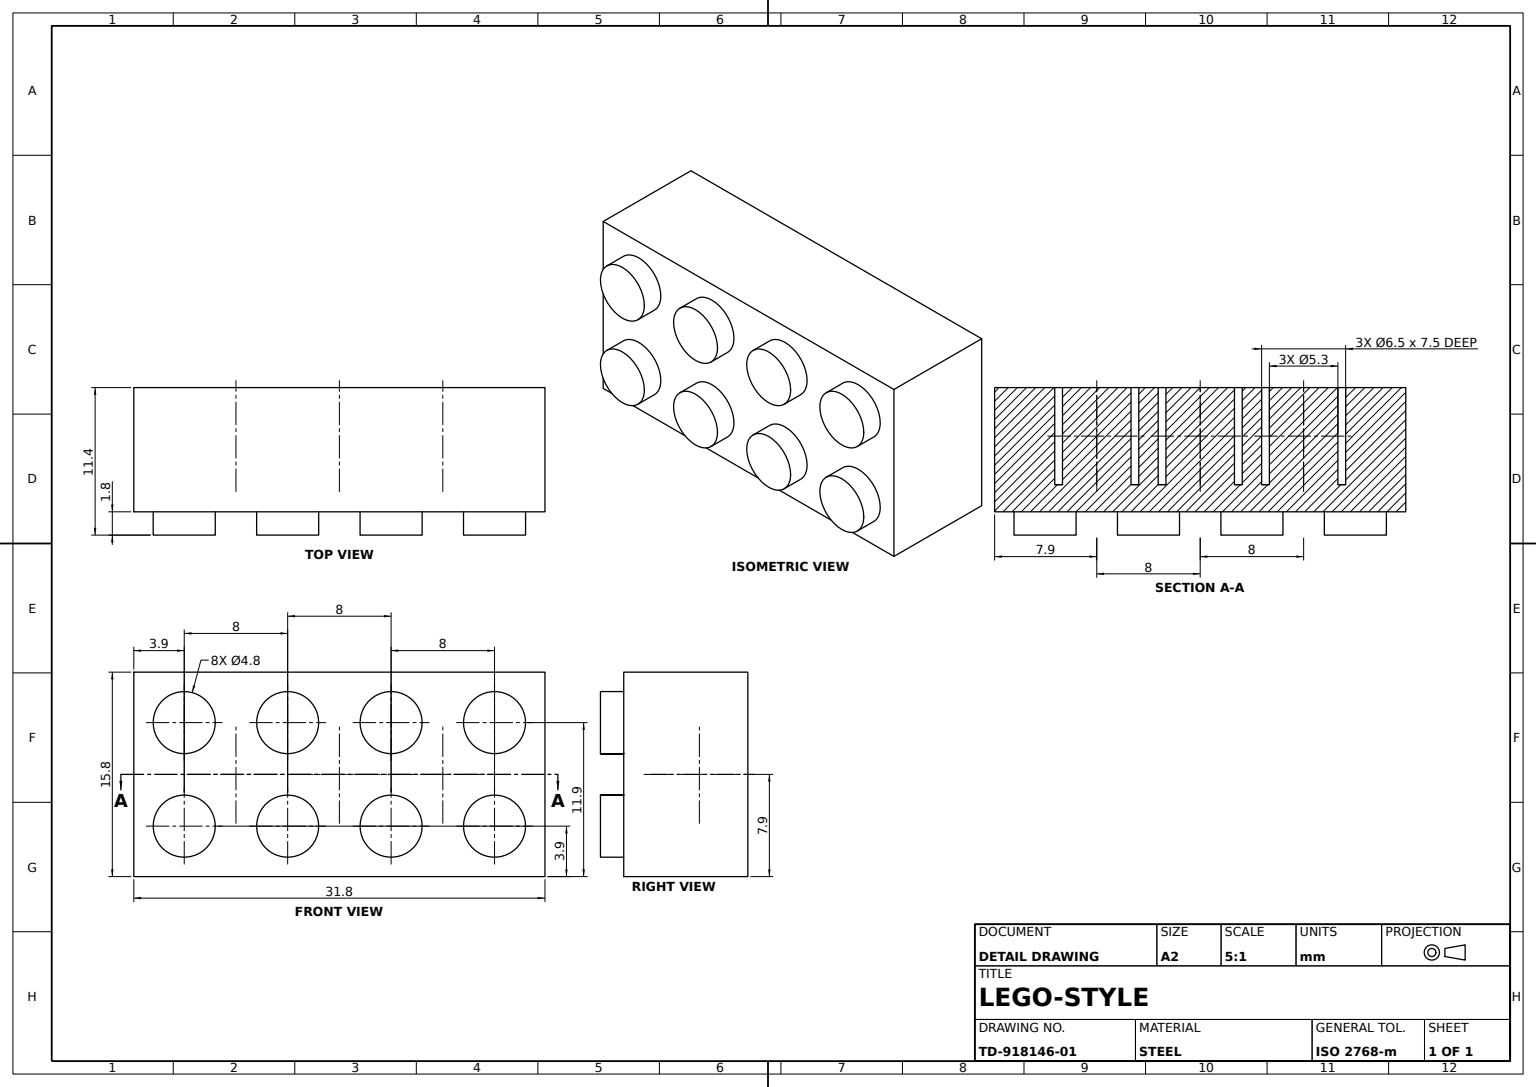
from build123d import *

# Parameters (mm, degrees)
BRICK_BODY_PROFILE_W         = 31.8
BRICK_BODY_PROFILE_H         = 15.8
BRICK_BODY_DEPTH             = 9.6
STUDS_PROFILE_2X4_4_8_R      = 2.4
STUDS_8X_4_8_DEPTH           = 1.8
UNDERSIDE_CAVITY_DEPTH       = 22.099289088
UNDERSIDE_CAVITY_DEPTH_BACK  = 7.5
UNDERSIDE_CAVITY_PROFILE_R   = 3.25
UNDERSIDE_CAVITY_PROFILE_R_2 = 2.65


with BuildPart() as part:
    # Brick Body Profile → Brick Body (new body)
    with BuildSketch(Plane.XY):
        Rectangle(BRICK_BODY_PROFILE_W, BRICK_BODY_PROFILE_H)
    extrude(amount=BRICK_BODY_DEPTH)

    # Studs Profile 2x4 Ø4.8 → Studs 8xØ4.8 (add)
    with BuildSketch(Plane.XY.offset(9.6)):
        with Locations((-12, 4)):
            Circle(STUDS_PROFILE_2X4_4_8_R)
        with Locations((-4, 4)):
            Circle(STUDS_PROFILE_2X4_4_8_R)
        with Locations((4, 4)):
            Circle(STUDS_PROFILE_2X4_4_8_R)
        with Locations((12, 4)):
            Circle(STUDS_PROFILE_2X4_4_8_R)
        with Locations(Location((12, -4, 0), (0, 0, 180))):
            Circle(STUDS_PROFILE_2X4_4_8_R)
        with Locations(Location((4, -4, 0), (0, 0, 180))):
            Circle(STUDS_PROFILE_2X4_4_8_R)
        with Locations(Location((-4, -4, 0), (0, 0, 180))):
            Circle(STUDS_PROFILE_2X4_4_8_R)
        with Locations(Location((-12, -4, 0), (0, 0, 180))):
            Circle(STUDS_PROFILE_2X4_4_8_R)
    extrude(amount=STUDS_8X_4_8_DEPTH)

    # Underside Cavity Profile → Underside Cavity (cut, two sides: drawn at the far end of the back side and taken through both)
    # profile 1 of 3: a face of its own
    with BuildSketch(Plane(origin=(0, 0, 0), x_dir=(-1, 0, 0), z_dir=(0, 0, -1)).offset(-UNDERSIDE_CAVITY_DEPTH_BACK)):
        with Locations(Location((-8, 0, 0), (0, 0, 180))):
            Circle(UNDERSIDE_CAVITY_PROFILE_R)
        with Locations(Location((-8, 0, 0), (0, 0, 180))):
            Circle(UNDERSIDE_CAVITY_PROFILE_R_2, mode=Mode.SUBTRACT)
    # profile 2 of 3: a face of its own
    with BuildSketch(Plane(origin=(0, 0, 0), x_dir=(-1, 0, 0), z_dir=(0, 0, -1)).offset(-UNDERSIDE_CAVITY_DEPTH_BACK)):
        with Locations(Location((0, 0, 0), (0, 0, 180))):
            Circle(UNDERSIDE_CAVITY_PROFILE_R)
        with Locations(Location((0, 0, 0), (0, 0, 180))):
            Circle(UNDERSIDE_CAVITY_PROFILE_R_2, mode=Mode.SUBTRACT)
    # profile 3 of 3: a face of its own
    with BuildSketch(Plane(origin=(0, 0, 0), x_dir=(-1, 0, 0), z_dir=(0, 0, -1)).offset(-UNDERSIDE_CAVITY_DEPTH_BACK)):
        with Locations(Location((8, 0, 0), (0, 0, 180))):
            Circle(UNDERSIDE_CAVITY_PROFILE_R)
        with Locations(Location((8, 0, 0), (0, 0, 180))):
            Circle(UNDERSIDE_CAVITY_PROFILE_R_2, mode=Mode.SUBTRACT)
    extrude(amount=UNDERSIDE_CAVITY_DEPTH + UNDERSIDE_CAVITY_DEPTH_BACK, mode=Mode.SUBTRACT)


solid = part.part
